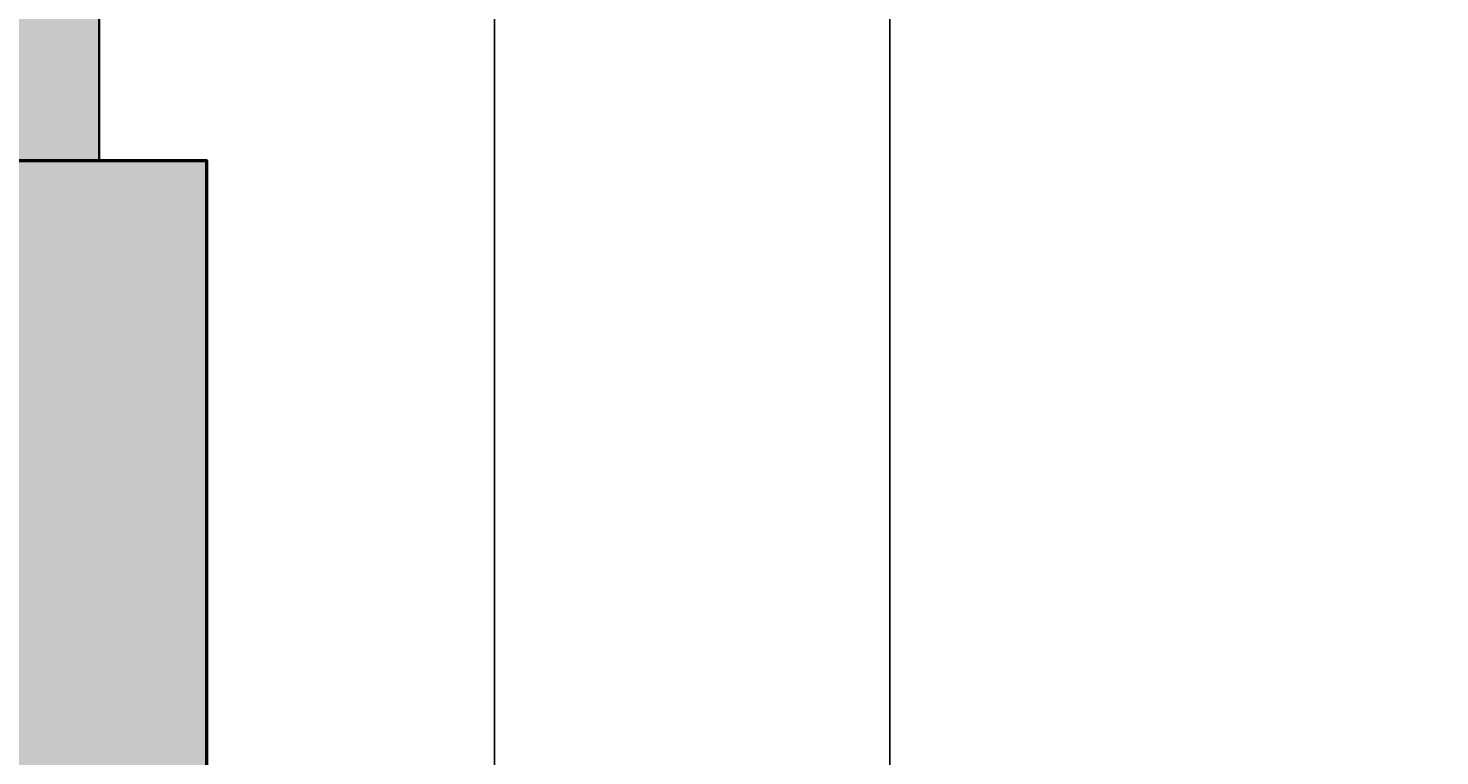
# Model space of a CAD drawing. Units: inches. Extents: x 1998 to 2588, y 1139 to 1977.
# Tile 62 of 134: x 2095 to 2127, y 1762 to 1779. Entities that reach past the tile are written whole.
import ezdxf

# ---------------------------------------------------------------- set-up
doc = ezdxf.new("R2010")
doc.units = ezdxf.units.IN
for name, color, linetype, lineweight in [('A-ANNO-DIMS', 2, 'Continuous', 18), ('A-COLS-PATT', 250, 'Continuous', 13), ('A-WALL-PATT', 252, 'Continuous', 13), ('COLUMN', 10, 'Continuous', 50), ('WALL', 200, 'Continuous', 35)]:
    doc.layers.add(name, color=color, linetype=linetype, lineweight=lineweight)
doc.styles.get("Standard").update_dxf_attribs({"font": 'arial.ttf'})
doc.dimstyles.get("Standard").update_dxf_attribs({"dimtxt": 0.18, "dimasz": 0.18, "dimexe": 0.18, "dimexo": 0.0625, "dimgap": 0.09, "dimtad": 0, "dimtih": 1, "dimtoh": 1, "dimdec": 4, "dimzin": 0, "dimdsep": 46, "dimtxsty": 'Standard', "dimcen": 0.09, "dimadec": 0, "dimazin": 0, "dimtfac": 1, "dimtdec": 4, "dimtofl": 0, "dimtmove": 0, "dimatfit": 3, "dimfxl": 1, "dimtolj": 1, "dimtzin": 0, "dimarcsym": 0})

# ---------------------------------------------------------------- blocks, each defined once
blk = doc.blocks.new('*D40')
at = {"layer": 'A-ANNO-DIMS', "color": 0, "lineweight": -2, "transparency": 16777216}
for p, q in [((2105.973, 1628.541), (2105.973, 1977.362)), ((2114.973, 1628.804), (2114.973, 1977.362)), ((2106.153, 1977.182), (2110.324, 1977.182)), ((2114.793, 1977.182), (2110.622, 1977.182))]:
    blk.add_line(p, q, dxfattribs=at)
at = {"layer": 'A-ANNO-DIMS', "color": 0, "transparency": 16777216}
for points in [[(2106.153, 1977.212), (2106.153, 1977.152), (2105.973, 1977.182)], [(2114.793, 1977.212), (2114.793, 1977.152), (2114.973, 1977.182)]]:
    blk.add_solid(points, dxfattribs=at)
at = {"layer": 'Defpoints', "color": 0, "transparency": 16777216}
for p in [(2114.973, 1977.182), (2114.973, 1628.742), (2105.973, 1628.478)]:
    blk.add_point(p, dxfattribs=at)
at = {"layer": 'A-ANNO-DIMS', "color": 0, "transparency": 16777216, "insert": (2110.473, 1977.182), "char_height": 0.18, "attachment_point": 5}
blk.add_mtext('\\A1;9', dxfattribs=at)

msp = doc.modelspace()

# ---------------------------------------------------------------- hatches: boundary and pattern name
at = {"layer": 'A-COLS-PATT'}
h = msp.add_hatch(color=256, dxfattribs=at)
h.dxf.hatch_style = 1
h.paths.add_polyline_path([(2099.4125, 1888.7324), (2087.9729, 1888.7324), (2087.9729, 1868.3278), (2099.4125, 1868.3278)])
h.paths.add_polyline_path([(2234.4125, 1888.7324), (2222.9729, 1888.7324), (2222.9729, 1868.3278), (2234.4125, 1868.3278)])
h.paths.add_polyline_path([(2341.4729, 1886.637), (2330.0332, 1886.637), (2330.0332, 1866.2324), (2341.4729, 1866.2324)])
h.paths.add_polyline_path([(2507.8006, 1882.7324), (2487.396, 1882.7324), (2487.396, 1871.2927), (2507.8006, 1871.2927)])
h.paths.add_polyline_path([(2510.9729, 1766.672), (2490.5682, 1766.672), (2490.5682, 1755.2324), (2510.9729, 1755.2324)])
h.paths.add_polyline_path([(2345.9729, 1759.7324), (2334.5332, 1759.7324), (2334.5332, 1739.3278), (2345.9729, 1739.3278)])
h.paths.add_polyline_path([(2234.4125, 1774.3318), (2222.9729, 1774.3318), (2222.9729, 1753.9272), (2234.4125, 1753.9272)])
h.paths.add_polyline_path([(2099.4125, 1775.637), (2087.9729, 1775.637), (2087.9729, 1755.2324), (2099.4125, 1755.2324)])
h.paths.add_polyline_path([(2098.0956, 1593.7241), (2077.691, 1593.7241), (2077.691, 1582.2845), (2098.0956, 1582.2845)])
h.paths.add_polyline_path([(2227.4729, 1604.637), (2216.0332, 1604.637), (2216.0332, 1584.2324), (2227.4729, 1584.2324)])
h.paths.add_polyline_path([(2345.9729, 1647.5211), (2334.5332, 1647.5211), (2334.5332, 1627.1165), (2345.9729, 1627.1165)])
h.paths.add_polyline_path([(2522.3775, 1641.2324), (2501.9729, 1641.2324), (2501.9729, 1629.7927), (2522.3775, 1629.7927)])
h.paths.add_polyline_path([(2522.3775, 1480.7324), (2501.9729, 1480.7324), (2501.9729, 1469.2927), (2522.3775, 1469.2927)])
h.paths.add_polyline_path([(2345.9729, 1488.5616), (2334.5332, 1488.5616), (2334.5332, 1468.1569), (2345.9729, 1468.1569)])
h.paths.add_polyline_path([(2234.4125, 1486.137), (2227.4729, 1486.137), (2227.4729, 1465.7324), (2234.4125, 1465.7324)])
h.paths.add_polyline_path([(2227.4729, 1486.137), (2222.9729, 1486.137), (2222.9729, 1465.7324), (2227.4729, 1465.7324)])
h.paths.add_polyline_path([(2108.3775, 1470.2324), (2087.9729, 1470.2324), (2087.9729, 1458.7927), (2108.3775, 1458.7927)])
h.paths.add_polyline_path([(2096.9729, 1365.5012), (2087.9729, 1365.5012), (2087.9729, 1345.0966), (2096.9729, 1345.0966)])
h.paths.add_polyline_path([(2087.9729, 1365.5012), (2085.5332, 1365.5012), (2085.5332, 1345.0966), (2087.9729, 1345.0966)])
h.paths.add_polyline_path([(2234.4125, 1285.137), (2222.9729, 1285.137), (2222.9729, 1264.7324), (2234.4125, 1264.7324)])
h.paths.add_polyline_path([(2345.9729, 1285.137), (2334.5332, 1285.137), (2334.5332, 1264.7324), (2345.9729, 1264.7324)])
h.paths.add_polyline_path([(2503.1458, 1240.172), (2482.7412, 1240.172), (2482.7412, 1228.7324), (2503.1458, 1228.7324)])
h.paths.add_polyline_path([(2510.9729, 1369.172), (2490.5682, 1369.172), (2490.5682, 1357.7324), (2510.9729, 1357.7324)])
at = {"layer": 'A-WALL-PATT'}
h = msp.add_hatch(color=256, dxfattribs=at)
h.dxf.hatch_style = 1
h.paths.add_polyline_path([(2222.9729, 1888.7324), (2099.4125, 1888.7324), (2099.4125, 1879.7324), (2222.9729, 1879.7324)])
h.paths.add_polyline_path([(2096.9729, 1868.3278), (2087.9729, 1868.3278), (2087.9729, 1775.637), (2096.9729, 1775.637)])
h.paths.add_polyline_path([(2227.4729, 1868.3278), (2222.9729, 1868.3278), (2222.9729, 1774.3318), (2227.4729, 1774.3318)])
h.paths.add_polyline_path([(2188.3019, 1759.7324), (2138.6074, 1759.7324), (2099.4125, 1759.7324), (2099.4125, 1755.2324), (2176.9729, 1755.2324), (2188.3019, 1755.2324)])
h.paths.add_polyline_path([(2087.9729, 1759.7324), (2059.4729, 1759.7324), (2059.4729, 1702.7324), (2087.9729, 1702.7324), (2087.9729, 1707.2324), (2063.9729, 1707.2324), (2063.9729, 1755.2324), (2087.9729, 1755.2324)])
h.paths.add_polyline_path([(2096.9729, 1755.2324), (2087.9729, 1755.2324), (2087.9729, 1707.2324), (2096.9729, 1707.2324)])
h.paths.add_polyline_path([(2187.0461, 1707.2324), (2105.9729, 1707.2324), (2096.9729, 1707.2324), (2087.9729, 1707.2324), (2087.9729, 1702.7324), (2105.9729, 1702.7324), (2114.9729, 1702.7324), (2187.0461, 1702.7324)])
h.paths.add_polyline_path([(2181.4729, 1719.2028), (2176.9729, 1719.2028), (2176.9729, 1707.2324), (2181.4729, 1707.2324)])
h.paths.add_polyline_path([(2216.0332, 1588.7324), (2114.9729, 1588.7324), (2105.9729, 1588.7324), (2105.9729, 1584.2324), (2216.0332, 1584.2324)])
h.paths.add_polyline_path([(2077.691, 1588.7324), (2061.4729, 1588.7324), (2061.4729, 1584.2324), (2077.691, 1584.2324)])
h.paths.add_polyline_path([(2105.9729, 1588.7324), (2098.0956, 1588.7324), (2098.0956, 1584.2324), (2105.9729, 1584.2324)])
h.paths.add_polyline_path([(2114.9729, 1596.2642), (2110.1012, 1596.2642), (2105.9729, 1596.2642), (2105.9729, 1588.7324), (2114.9729, 1588.7324)])
h.paths.add_polyline_path([(2114.9729, 1584.2324), (2105.9729, 1584.2324), (2105.9729, 1580.249), (2110.1012, 1580.249), (2114.9729, 1580.249)])
h.paths.add_polyline_path([(2114.9729, 1547.7716), (2110.1012, 1547.7716, -0.0318759), (2105.9729, 1548.035), (2105.9729, 1470.2324), (2108.3775, 1470.2324), (2108.3775, 1465.7324), (2186.2943, 1465.7324), (2186.2943, 1470.2324), (2114.9729, 1470.2324)])
h.paths.add_polyline_path([(2227.4729, 1584.2324), (2222.9729, 1584.2324), (2222.9729, 1486.137), (2227.4729, 1486.137)])
h.paths.add_polyline_path([(2295.4138, 1593.2324), (2227.4729, 1593.2324), (2227.4729, 1588.7324), (2295.4138, 1588.7324), (2295.4138, 1591.8729)])
h.paths.add_polyline_path([(2345.9729, 1627.1165), (2341.4729, 1627.1165), (2341.4729, 1593.2324), (2337.2869, 1593.2324), (2337.2869, 1591.8729), (2337.2869, 1588.7324), (2345.9729, 1588.7324)])
h.paths.add_polyline_path([(2291.9729, 1588.7324), (2287.4729, 1588.7324), (2287.4729, 1522.7324), (2291.9729, 1522.7324)])
h.paths.add_polyline_path([(2291.9729, 1522.7324), (2287.4729, 1522.7324), (2227.4729, 1522.7324), (2227.4729, 1518.2324), (2291.9729, 1518.2324)])
h.paths.add_polyline_path([(2295.7347, 1519.5919), (2295.7347, 1522.7324), (2291.9729, 1522.7324), (2291.9729, 1518.2324), (2295.7347, 1518.2324)])
h.paths.add_polyline_path([(2345.9729, 1522.7324), (2337.6078, 1522.7324), (2337.6078, 1519.5919), (2337.6078, 1518.2324), (2341.4729, 1518.2324), (2341.4729, 1488.5616), (2345.9729, 1488.5616)])
h.paths.add_polyline_path([(2345.9729, 1468.1569), (2341.4729, 1468.1569), (2341.4729, 1374.2324), (2227.4729, 1374.2324), (2227.4729, 1369.7324), (2345.9729, 1369.7324)])
h.paths.add_polyline_path([(2345.9729, 1369.7324), (2341.4729, 1369.7324), (2341.4729, 1362.2324), (2345.9729, 1362.2324)])
h.paths.add_polyline_path([(2345.9729, 1317.7324), (2345.9729, 1322.2324), (2341.4729, 1322.2324), (2341.4729, 1285.137), (2345.9729, 1285.137)], flags=17)
h.paths.add_polyline_path([(2356.2096, 1322.2324), (2345.9729, 1322.2324), (2345.9729, 1317.7324), (2356.2096, 1317.7324), (2356.2096, 1319.3088)], flags=17)
h.paths.add_polyline_path([(2393.9729, 1322.2324), (2375.6999, 1322.2324), (2375.6999, 1319.3088, -0.0202458), (2375.636, 1317.7324), (2393.9729, 1317.7324)], flags=17)
h.paths.add_polyline_path([(2398.4729, 1322.2324), (2393.9729, 1322.2324), (2393.9729, 1317.7324), (2393.9729, 1237.7324), (2345.9729, 1237.7324), (2345.9729, 1264.7324), (2341.4729, 1264.7324), (2341.4729, 1228.7324), (2393.9729, 1228.7324), (2482.7412, 1228.7324), (2482.7412, 1237.7324), (2398.4729, 1237.7324), (2398.4729, 1297.1029)])
h.paths.add_polyline_path([(2398.4729, 1362.2324), (2393.9729, 1362.2324), (2393.9729, 1357.7324), (2398.4729, 1357.7324)])
h.paths.add_polyline_path([(2345.9729, 1329.7549), (2341.4729, 1329.7549), (2341.4729, 1322.2324), (2345.9729, 1322.2324)])

# ---------------------------------------------------------------- linework, layer by layer
at = {"layer": 'COLUMN'}
msp.add_lwpolyline([(2087.9729, 1775.637), (2099.4125, 1775.637), (2099.4125, 1755.2324), (2087.9729, 1755.2324)], close=True, dxfattribs=at)
at = {"layer": 'WALL'}
msp.add_line((2096.9729, 1868.3278), (2096.9729, 1775.637), dxfattribs=at)

# ---------------------------------------------------------------- dimensions: what is measured, and where the dimension line sits
at = {"layer": 'A-ANNO-DIMS'}
dim = msp.add_linear_dim(base=(2114.9729, 1977.1824), p1=(2105.9729, 1628.4781), p2=(2114.9729, 1628.7416), dimstyle='Standard', override={"dimdec": 0, "dimlfac": 1, "dimrnd": 0, "dimzin": 0, "dimdsep": 46, "dimlunit": 2}, dxfattribs=at)
dim.commit()
dim.dimension.update_dxf_attribs({"geometry": '*D40', "text_midpoint": (2110.4729, 1977.1824)})

doc.saveas('drawing.dxf')
